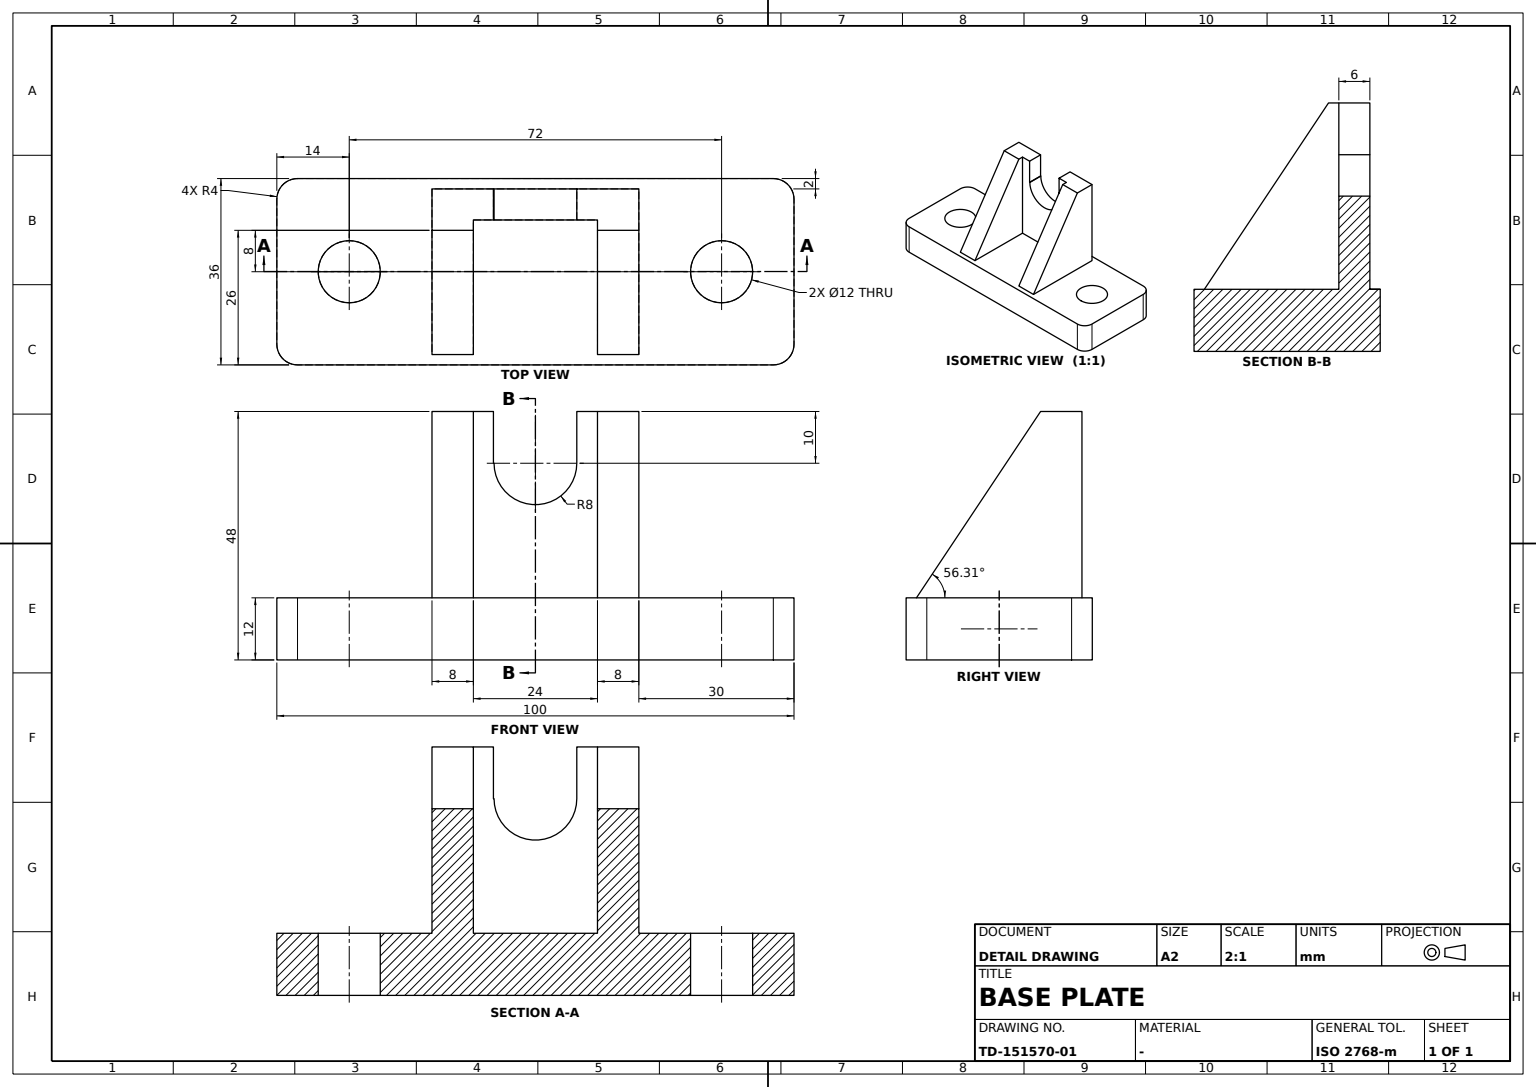
CATIA V5 part; units mm, degrees
sketch "Sketch1" plane through (0, 0, 0) normal (0, 0, 1) x (0, 1, 0)
  line L0 (0, 0) -> (100, 0)
  line L1 (100, 0) -> (100, -36)
  line L2 (100, -36) -> (0, -36)
  line L3 (0, -36) -> (0, 0)
  dimension "length L1" = 36
  dimension "length L2" = 100
  constraint horizontal L0 x-axis
  constraint horizontal L2 x-axis
  constraint vertical L1 y-axis
  constraint vertical L3 y-axis
extrude "Pad1" add sketch "Sketch1" along normal blind 12
sketch "Sketch2" plane through (0, 100, 0) normal (0, 1, 0) x (-1, 0, 0)
  line L0 (-2, 12) -> (-2, 48)
  line L1 (-2, 48) -> (-10, 48)
  line L2 (-10, 48) -> (-34, 12)
  point P0 (-34, 12)
  line L3 (-34, 12) -> (-2, 12)
  line L4 (-36, 12) -> (0, 12) construction
  line L5 (-36, 0) -> (-36, 12) construction
  dimension "length L0" = 36
  dimension "D2" = 2
  dimension "length L1" = 8
  dimension "distance P0 L5" = 2
  constraint vertical L0 y-axis
  constraint horizontal L1 x-axis
  constraint horizontal L3 x-axis
  constraint coincidence L3 L4
extrude "Pad2" add sketch "Sketch2" against normal blind 100
sketch "Sketch3" plane through (0, 100, 0) normal (0, 1, 0) x (-1, 0, 0)
  line L0 (-34.1651, 12) -> (-2, 12)
  line L1 (-2, 12) -> (-2, 48.4282)
  line L2 (-2, 48.4282) -> (-9.8317, 48.4282)
  line L3 (-9.8317, 48.4282) -> (-34.1651, 12)
  constraint horizontal L0 x-axis
  constraint horizontal L2 x-axis
  constraint vertical L1 y-axis
extrude "Pocket1" cut sketch "Sketch3" against normal blind 30
sketch "Sketch4" plane through (2, 0, 0) normal (-1, 0, 0) x (0, -1, 0)
  point P0 (0, 12)
  line L0 (0, 12) -> (-30, 12)
  line L1 (-30, 12) -> (-30, 48)
  line L2 (-30, 48) -> (0, 48)
  line L3 (0, 48) -> (0, 12)
  dimension "length L2" = 30
  constraint coincidence P0 y-axis
  constraint horizontal L0 x-axis
  constraint horizontal L2 x-axis
  constraint vertical L1 y-axis
  constraint vertical L3 y-axis
extrude "Pocket2" cut sketch "Sketch4" against normal blind 36
sketch "Sketch5" plane through (0, 0, 48) normal (0, 0, 1) x (1, 0, 0)
  line L0 (8, 62) -> (34, 62)
  line L1 (34, 62) -> (34, 38)
  line L2 (34, 38) -> (8, 38)
  line L3 (8, 38) -> (8, 62)
  line L4 (34, 100) -> (34, 0) construction
  line L5 (34, 70) -> (10, 70) construction
  dimension "length L0" = 26
  dimension "length L3" = 24
  dimension "distance L5 L0" = 8
  constraint horizontal L0 x-axis
  constraint horizontal L2 x-axis
  constraint vertical L1 y-axis
  constraint vertical L3 y-axis
  constraint coincidence L1 L4
extrude "Pocket3" cut sketch "Sketch5" against normal blind 36
sketch "Sketch6" plane through (2, 0, 0) normal (-1, 0, 0) x (0, -1, 0)
  arc A0 (-58, 38) -> (-42, 38) centre (-50, 38) ccw
  point P0 (-50, 38)
  line L0 (-100, 48) -> (0, 48) construction
  line L1 (-30, 48) -> (-30, 12) construction
  line L2 (-42, 38) -> (-41.8797, 38)
  line L3 (-41.8797, 38) -> (-41.8797, 48.237)
  line L4 (-41.8797, 48.237) -> (-58, 48.237)
  line L5 (-58, 48.237) -> (-58, 38)
  dimension "radius A0" = 8
  dimension "distance P0 L0" = 10
  dimension "distance P0 L1" = 20
  constraint horizontal L2 x-axis
  constraint horizontal L4 x-axis
  constraint vertical L3 y-axis
  constraint vertical L5 y-axis
extrude "Pocket4" cut sketch "Sketch6" against normal up to next
sketch "Sketch7" plane through (0, 0, 12) normal (0, 0, 1) x (1, 0, 0)
  circle A0 centre (18, 14) radius 6
  point P0 (18, 14)
  line L0 (36, 0) -> (36, 100) construction
  line L1 (0, 0) -> (36, 0) construction
  circle A1 centre (18, 86) radius 6
  point P1 (18, 86)
  dimension "radius A0" = 6
  dimension "distance P0 L0" = 18
  dimension "distance P0 L1" = 14
  dimension "radius A1" = 6
  dimension "distance P1 P0" = 72
extrude "Pocket5" cut sketch "Sketch7" against normal up to next
fillet "Fillet1" radius 4 4 edges at (36, 100, 6) (0, 100, 6) (36, 0, 6) (0, 0, 6)
properties part number "catia 21"
